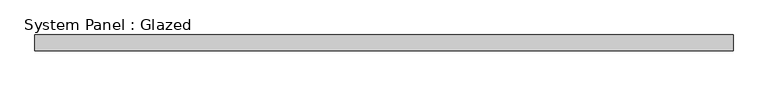
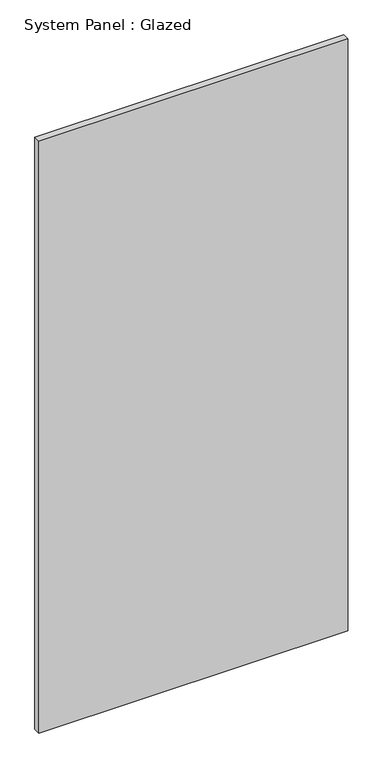
"""IFC4 building model written with IfcOpenShell, lengths in millimetres: plate geometry, System Panel : Glazed."""

from ifc_helpers import new_model, si_unit, origin, origin_with_axes, place, context, project, spatial, polyline, outline, extrude, source, transform, mapped, element, save


def system_panel_glazed_a1d10a75(model_context):
    return source(origin(), model_context, "Body", "SweptSolid", [
        extrude(outline(polyline([(568.3249999, 19.05), (-568.3249999, 19.05), (-568.3249999, 44.45), (568.3249999, 44.45), (568.3249999, 19.05)])), origin_with_axes(), (0.0, 0.0, 1.0), 2301.9640157),
    ])


if __name__ == "__main__":
    model = new_model("IFC4")
    model_context = context("Model", 3, world=origin())
    ifc_project = project(units=[si_unit("LENGTHUNIT", "METRE", prefix="MILLI")], contexts=[model_context])
    site = spatial("IfcSite", under=ifc_project)
    building = spatial("IfcBuilding", under=site)
    placement = place(None, origin())
    system_panel_glazed_shape = system_panel_glazed_a1d10a75(model_context)
    element("IfcPlate", 1, ObjectType="System Panel : Glazed", at=placement, inside=building, context=model_context, shape_type="MappedRepresentation", body=[
        mapped(system_panel_glazed_shape, transform((0.0, 0.0, 0.0), x_axis=(1.0, 0.0, 0.0), y_axis=(0.0, 1.0, 0.0), z_axis=(0.0, 0.0, 1.0))),
    ])
    save(model, "model.ifc")

# Revit data of these elements
# Type "System Panel : Glazed"
#   Construction Type Id = "GSP4R"
#   Analytic Construction = "1/8 in Pilkington single glazing"
#   Visual Light Transmittance = 0.9
#   Solar Heat Gain Coefficient = 0.86
#   Heat Transfer Coefficient (U) = 1.18115 BTU/(h·ft²·°F)
#   Define Thermal Properties by = 1
# Element 1 (IfcPlate, "System Panel : Glazed")
#   Materials on its faces: "Glass"
# Materials
#   "Glass": class "Glass", colour RGB 0 128 192, transparency 0.75, Description = "Soda Lime Glass", Cost = 0
